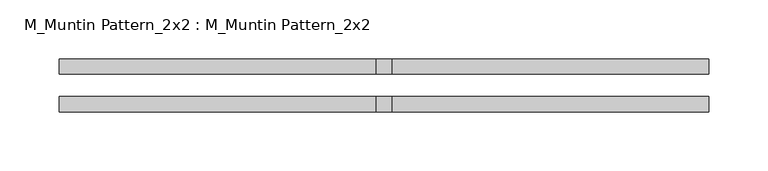
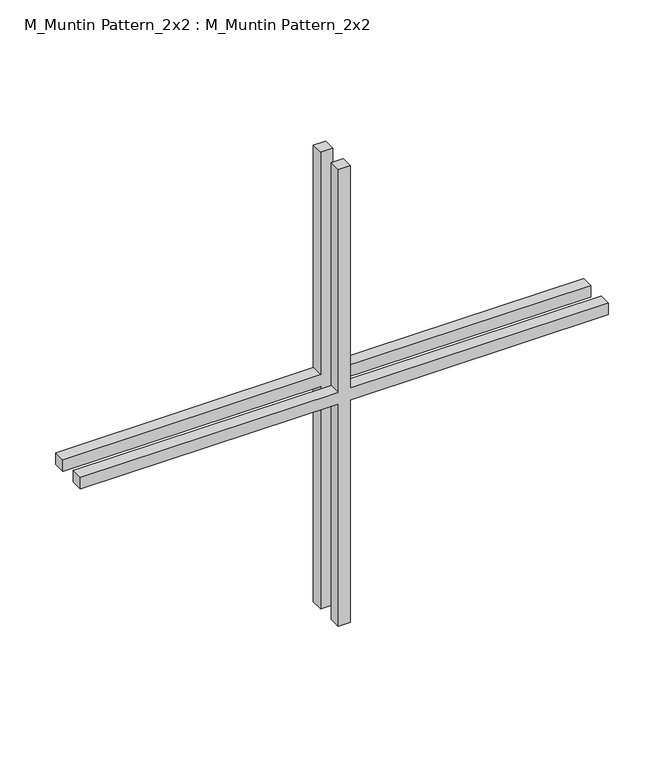
"""IFC4 building model written with IfcOpenShell, lengths in millimetres: proxy geometry, M_Muntin Pattern_2x2 : M_Muntin Pattern_2x2."""

from ifc_helpers import new_model, si_unit, frame, origin, place, context, project, spatial, polyline, outline, extrude, source, transform, mapped, element, save


def m_muntin_pattern_2x2_m_muntin_pattern_2x2_8c828626(model_context):
    return source(origin(), model_context, "Body", "SweptSolid", [
        extrude(outline(polyline([(257.1375, -6.35), (257.1375, -273.8), (244.4375, -273.8), (244.4375, -6.35), (0.0, -6.35), (0.0, 6.35), (244.4375, 6.35), (244.4375, 273.8), (257.1375, 273.8), (257.1375, 6.35), (501.575, 6.35), (501.575, -6.35), (257.1375, -6.35)])), frame((0.0, 9.525, 0.0), z_axis=(0.0, 1.0, 0.0), x_axis=(0.0, 0.0, 1.0)), (0.0, 0.0, 1.0), 12.7),
        extrude(outline(polyline([(257.1375, -6.35), (257.1375, -273.8), (244.4375, -273.8), (244.4375, -6.35), (0.0, -6.35), (0.0, 6.35), (244.4375, 6.35), (244.4375, 273.8), (257.1375, 273.8), (257.1375, 6.35), (501.575, 6.35), (501.575, -6.35), (257.1375, -6.35)])), frame((0.0, -22.225, 0.0), z_axis=(0.0, 1.0, 0.0), x_axis=(0.0, 0.0, 1.0)), (0.0, 0.0, 1.0), 12.7),
    ])


if __name__ == "__main__":
    model = new_model("IFC4")
    model_context = context("Model", 3, world=origin())
    ifc_project = project(units=[si_unit("LENGTHUNIT", "METRE", prefix="MILLI")], contexts=[model_context])
    site = spatial("IfcSite", under=ifc_project)
    building = spatial("IfcBuilding", under=site)
    placement = place(None, origin())
    m_muntin_pattern_2x2_m_muntin_pattern_2x2_shape = m_muntin_pattern_2x2_m_muntin_pattern_2x2_8c828626(model_context)
    element("IfcBuildingElementProxy", 1, Name="M_Muntin Pattern_2x2 : M_Muntin Pattern_2x2", ObjectType="M_Muntin Pattern_2x2 : M_Muntin Pattern_2x2", at=placement, inside=building, context=model_context, shape_type="MappedRepresentation", body=[
        mapped(m_muntin_pattern_2x2_m_muntin_pattern_2x2_shape, transform((0.0, 0.0, 0.0), x_axis=(1.0, 0.0, 0.0), y_axis=(0.0, 1.0, 0.0), z_axis=(0.0, 0.0, 1.0))),
    ])
    save(model, "model.ifc")

# Revit data of these elements
# Type "M_Muntin Pattern_2x2 : M_Muntin Pattern_2x2"
#   Width [instance default] = 1.2 m
#   Thickness = 0.0127 m
#   Height [instance default] = 1.2 m
#   Distance = 0.01905 m
#   Interior Material [instance default] = none
#   Exterior Material [instance default] = none
#   Default Elevation = 0
# Element 1 (IfcBuildingElementProxy, "M_Muntin Pattern_2x2 : M_Muntin Pattern_2x2")
#   Width = 0.5476 m
#   Height = 0.501575 m
#   Interior Material = Wood - Stained
#   Exterior Material = Clad - White
#   Materials on its faces: "Clad - White", "Wood - Stained"
# Materials
#   "Clad - White": class "Wood", colour RGB 242 242 238, transparency 0, Cost = 0
#   "Wood - Stained": class "Wood", colour RGB 224 178 126, transparency 0, Cost = 0
